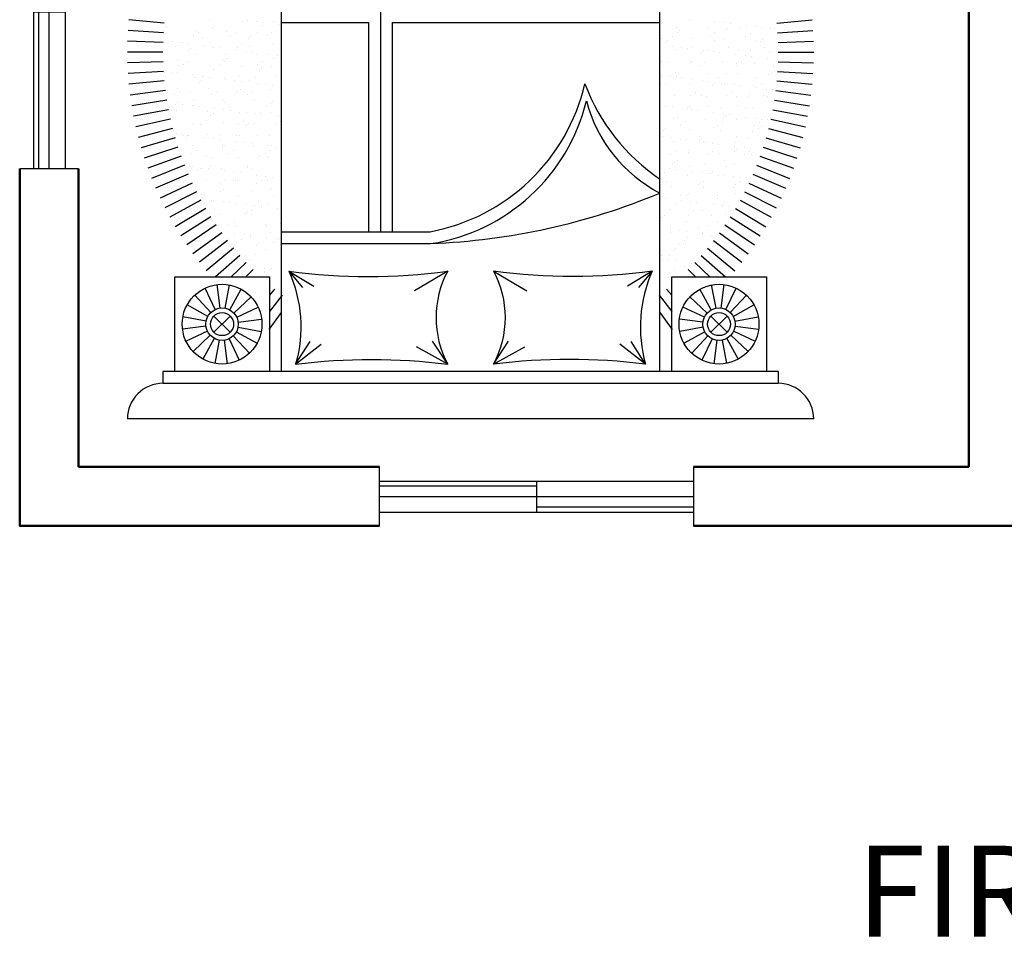
# Model space of a CAD drawing. Units: millimetres. Extents: x -857 to 54106, y -13666 to 13947.
# Tile 13 of 41: x 21020 to 24780, y 2329 to 5837. Entities that reach past the tile are written whole.
import ezdxf

# ---------------------------------------------------------------- set-up
doc = ezdxf.new("R2010")
doc.units = ezdxf.units.MM
for name, color, linetype, lineweight in [('A-ANNO-TEXT', 7, 'Continuous', 25), ('A-FURN', 21, 'Continuous', 18), ('A-GLAZ', 4, 'Continuous', 25), ('A-WALL', 7, 'Continuous', 50)]:
    doc.layers.add(name, color=color, linetype=linetype, lineweight=lineweight)
for name, color, linetype in [('A-FRN', 11, 'Continuous'), ('A-HT', 15, 'Continuous'), ('L-HT', 1, 'Continuous')]:
    doc.layers.add(name, color=color, linetype=linetype)
doc.styles.get("Standard").update_dxf_attribs({"font": 'arial.ttf'})

# ---------------------------------------------------------------- blocks, each defined once
blk = doc.blocks.new('*X18')
at = {"color": 0}
for p, q in [((0.9013, 1.6721), (0.9013, 1.6721)), ((0.9273, 1.6756), (0.9273, 1.6756)), ((0.9679, 1.6809), (0.9679, 1.6809)), ((1.075, 1.6828), (1.075, 1.6828)), ((2.8098, 1.6645), (2.8098, 1.6645)), ((2.8341, 1.6809), (2.8341, 1.6809)), ((2.8777, 1.6734), (2.8777, 1.6734)), ((2.9037, 1.6769), (2.9037, 1.6769)), ((2.9444, 1.6822), (2.9444, 1.6822)), ((2.962, 1.6803), (2.962, 1.6803)), ((3.0971, 1.6852), (3.0971, 1.6852)), ((0.7154, 1.6491), (0.7154, 1.6491)), ((0.7341, 1.6496), (0.7341, 1.6496)), ((0.7667, 1.6544), (0.7667, 1.6544)), ((0.7927, 1.6578), (0.7927, 1.6578)), ((0.8149, 1.6302), (0.8149, 1.6302)), ((0.8333, 1.6632), (0.8333, 1.6632)), ((0.865, 1.6513), (0.865, 1.6513)), ((0.9155, 1.6474), (0.9155, 1.6474)), ((0.9247, 1.6389), (0.9247, 1.6389)), ((0.9706, 1.6305), (0.9706, 1.6305)), ((0.9929, 1.6507), (0.9929, 1.6507)), ((1.1185, 1.6429), (1.1185, 1.6429)), ((1.1263, 1.6308), (1.1263, 1.6308)), ((1.1279, 1.6556), (1.1279, 1.6556)), ((2.8391, 1.6339), (2.8391, 1.6339)), ((2.8812, 1.6623), (2.8812, 1.6623)), ((2.9017, 1.634), (2.9017, 1.634)), ((2.9948, 1.6342), (2.9948, 1.6342)), ((3.0326, 1.6357), (3.0326, 1.6357)), ((3.0813, 1.6605), (3.0813, 1.6605)), ((3.0905, 1.6521), (3.0905, 1.6521)), ((3.1505, 1.6345), (3.1505, 1.6345)), ((3.1605, 1.6351), (3.1605, 1.6351)), ((3.2843, 1.6561), (3.2843, 1.6561)), ((3.2956, 1.64), (3.2956, 1.64)), ((0.7652, 1.6035), (0.7652, 1.6035)), ((0.7744, 1.595), (0.7744, 1.595)), ((0.7976, 1.5996), (0.7976, 1.5996)), ((0.836, 1.6168), (0.836, 1.6168)), ((0.9326, 1.6044), (0.9326, 1.6044)), ((0.9682, 1.599), (0.9682, 1.599)), ((0.9917, 1.6171), (0.9917, 1.6171)), ((1.0635, 1.6061), (1.0635, 1.6061)), ((1.1474, 1.6173), (1.1474, 1.6173)), ((1.1683, 1.5973), (1.1683, 1.5973)), ((1.1775, 1.5889), (1.1775, 1.5889)), ((1.1914, 1.6055), (1.1914, 1.6055)), ((2.8373, 1.5846), (2.8373, 1.5846)), ((2.8602, 1.6205), (2.8602, 1.6205)), ((2.931, 1.6167), (2.931, 1.6167)), ((2.9402, 1.6082), (2.9402, 1.6082)), ((2.9652, 1.584), (2.9652, 1.584)), ((3.0159, 1.6207), (3.0159, 1.6207)), ((3.1002, 1.5888), (3.1002, 1.5888)), ((3.134, 1.6122), (3.134, 1.6122)), ((3.1716, 1.621), (3.1716, 1.621)), ((3.193, 1.5855), (3.193, 1.5855)), ((3.219, 1.5889), (3.219, 1.5889)), ((3.2311, 1.5905), (3.2311, 1.5905)), ((3.2596, 1.5943), (3.2596, 1.5943)), ((0.7373, 1.5533), (0.7373, 1.5533)), ((0.7562, 1.5681), (0.7562, 1.5681)), ((0.8179, 1.5552), (0.8179, 1.5552)), ((0.8681, 1.555), (0.8681, 1.555)), ((0.8794, 1.5398), (0.8794, 1.5398)), ((0.9119, 1.5684), (0.9119, 1.5684)), ((0.9474, 1.5488), (0.9474, 1.5488)), ((0.9734, 1.5522), (0.9734, 1.5522)), ((0.996, 1.5544), (0.996, 1.5544)), ((1.014, 1.5575), (1.014, 1.5575)), ((1.018, 1.5534), (1.018, 1.5534)), ((1.0272, 1.545), (1.0272, 1.545)), ((1.0676, 1.5687), (1.0676, 1.5687)), ((1.0819, 1.5665), (1.0819, 1.5665)), ((1.108, 1.5699), (1.108, 1.5699)), ((1.1311, 1.5592), (1.1311, 1.5592)), ((1.1486, 1.5753), (1.1486, 1.5753)), ((2.8559, 1.5411), (2.8559, 1.5411)), ((2.9238, 1.55), (2.9238, 1.55)), ((2.9361, 1.5721), (2.9361, 1.5721)), ((2.9498, 1.5535), (2.9498, 1.5535)), ((2.9837, 1.5683), (2.9837, 1.5683)), ((2.9905, 1.5588), (2.9905, 1.5588)), ((3.0584, 1.5678), (3.0584, 1.5678)), ((3.0844, 1.5712), (3.0844, 1.5712)), ((3.0918, 1.5724), (3.0918, 1.5724)), ((3.1251, 1.5765), (3.1251, 1.5765)), ((3.1838, 1.5666), (3.1838, 1.5666)), ((3.193, 1.5582), (3.193, 1.5582)), ((3.2475, 1.5727), (3.2475, 1.5727)), ((3.2987, 1.5436), (3.2987, 1.5436)), ((0.7042, 1.5167), (0.7042, 1.5167)), ((0.7448, 1.5221), (0.7448, 1.5221)), ((0.8007, 1.5032), (0.8007, 1.5032)), ((0.8128, 1.531), (0.8128, 1.531)), ((0.8388, 1.5345), (0.8388, 1.5345)), ((0.8553, 1.505), (0.8553, 1.505)), ((0.8677, 1.5096), (0.8677, 1.5096)), ((0.8769, 1.5011), (0.8769, 1.5011)), ((0.9358, 1.5081), (0.9358, 1.5081)), ((1.011, 1.5053), (1.011, 1.5053)), ((1.0666, 1.5098), (1.0666, 1.5098)), ((1.0707, 1.5051), (1.0707, 1.5051)), ((1.1667, 1.5056), (1.1667, 1.5056)), ((1.1945, 1.5091), (1.1945, 1.5091)), ((2.8152, 1.5357), (2.8152, 1.5357)), ((2.8334, 1.5245), (2.8334, 1.5245)), ((2.8795, 1.5087), (2.8795, 1.5087)), ((2.9049, 1.5377), (2.9049, 1.5377)), ((3.0334, 1.5227), (3.0334, 1.5227)), ((3.0352, 1.509), (3.0352, 1.509)), ((3.0358, 1.5394), (3.0358, 1.5394)), ((3.0427, 1.5143), (3.0427, 1.5143)), ((3.1637, 1.5388), (3.1637, 1.5388)), ((3.1909, 1.5093), (3.1909, 1.5093)), ((3.2365, 1.5183), (3.2365, 1.5183)), ((0.7174, 1.4657), (0.7174, 1.4657)), ((0.7207, 1.4913), (0.7207, 1.4913)), ((0.7266, 1.4572), (0.7266, 1.4572)), ((0.7404, 1.457), (0.7404, 1.457)), ((0.8713, 1.4586), (0.8713, 1.4586)), ((0.8764, 1.4916), (0.8764, 1.4916)), ((0.9204, 1.4613), (0.9204, 1.4613)), ((0.9992, 1.458), (0.9992, 1.458)), ((1.0321, 1.4919), (1.0321, 1.4919)), ((1.1205, 1.4595), (1.1205, 1.4595)), ((1.1342, 1.4629), (1.1342, 1.4629)), ((1.1878, 1.4921), (1.1878, 1.4921)), ((2.8404, 1.4882), (2.8404, 1.4882)), ((2.8831, 1.4789), (2.8831, 1.4789)), ((2.8924, 1.4704), (2.8924, 1.4704)), ((2.9006, 1.4953), (2.9006, 1.4953)), ((2.9683, 1.4876), (2.9683, 1.4876)), ((3.0563, 1.4955), (3.0563, 1.4955)), ((3.0862, 1.4744), (3.0862, 1.4744)), ((3.1034, 1.4925), (3.1034, 1.4925)), ((3.212, 1.4958), (3.212, 1.4958)), ((3.2343, 1.4942), (3.2343, 1.4942)), ((3.2391, 1.4621), (3.2391, 1.4621)), ((3.2651, 1.4655), (3.2651, 1.4655)), ((3.2862, 1.4727), (3.2862, 1.4727)), ((3.2954, 1.4643), (3.2954, 1.4643)), ((0.7701, 1.4174), (0.7701, 1.4174)), ((0.7966, 1.4429), (0.7966, 1.4429)), ((0.9255, 1.4164), (0.9255, 1.4164)), ((0.9523, 1.4432), (0.9523, 1.4432)), ((0.9701, 1.4157), (0.9701, 1.4157)), ((0.9935, 1.4254), (0.9935, 1.4254)), ((1.0195, 1.4288), (1.0195, 1.4288)), ((1.0601, 1.4341), (1.0601, 1.4341)), ((1.108, 1.4435), (1.108, 1.4435)), ((1.128, 1.4431), (1.128, 1.4431)), ((1.1297, 1.4511), (1.1297, 1.4511)), ((1.1541, 1.4465), (1.1541, 1.4465)), ((1.1947, 1.4519), (1.1947, 1.4519)), ((2.8208, 1.4466), (2.8208, 1.4466)), ((2.902, 1.4177), (2.902, 1.4177)), ((2.908, 1.4414), (2.908, 1.4414)), ((2.9359, 1.4306), (2.9359, 1.4306)), ((2.9699, 1.4267), (2.9699, 1.4267)), ((2.9765, 1.4469), (2.9765, 1.4469)), ((2.9959, 1.4301), (2.9959, 1.4301)), ((3.0366, 1.4354), (3.0366, 1.4354)), ((3.0389, 1.443), (3.0389, 1.443)), ((3.1045, 1.4444), (3.1045, 1.4444)), ((3.1305, 1.4478), (3.1305, 1.4478)), ((3.1322, 1.4472), (3.1322, 1.4472)), ((3.1359, 1.4288), (3.1359, 1.4288)), ((3.1451, 1.4204), (3.1451, 1.4204)), ((3.1668, 1.4424), (3.1668, 1.4424)), ((3.1712, 1.4532), (3.1712, 1.4532)), ((3.2879, 1.4475), (3.2879, 1.4475)), ((0.7243, 1.3899), (0.7243, 1.3899)), ((0.74, 1.3795), (0.74, 1.3795)), ((0.7503, 1.3934), (0.7503, 1.3934)), ((0.7909, 1.3987), (0.7909, 1.3987)), ((0.8039, 1.4069), (0.8039, 1.4069)), ((0.8589, 1.4076), (0.8589, 1.4076)), ((0.8849, 1.4111), (0.8849, 1.4111)), ((0.8957, 1.3798), (0.8957, 1.3798)), ((0.9389, 1.4118), (0.9389, 1.4118)), ((0.9794, 1.4072), (0.9794, 1.4072)), ((1.0514, 1.3801), (1.0514, 1.3801)), ((1.0698, 1.4134), (1.0698, 1.4134)), ((1.1732, 1.4112), (1.1732, 1.4112)), ((1.1977, 1.4128), (1.1977, 1.4128)), ((2.8353, 1.4089), (2.8353, 1.4089)), ((2.8436, 1.3919), (2.8436, 1.3919)), ((2.8613, 1.4124), (2.8613, 1.4124)), ((2.9199, 1.3835), (2.9199, 1.3835)), ((2.9715, 1.3913), (2.9715, 1.3913)), ((2.9856, 1.385), (2.9856, 1.385)), ((2.9948, 1.3765), (2.9948, 1.3765)), ((3.0756, 1.3838), (3.0756, 1.3838)), ((3.1065, 1.3961), (3.1065, 1.3961)), ((3.1886, 1.3805), (3.1886, 1.3805)), ((3.2313, 1.384), (3.2313, 1.384)), ((3.2374, 1.3978), (3.2374, 1.3978)), ((0.7436, 1.3606), (0.7436, 1.3606)), ((0.761, 1.3661), (0.761, 1.3661)), ((0.8198, 1.3718), (0.8198, 1.3718)), ((0.8291, 1.3633), (0.8291, 1.3633)), ((0.8744, 1.3623), (0.8744, 1.3623)), ((0.9168, 1.3664), (0.9168, 1.3664)), ((1.0023, 1.3617), (1.0023, 1.3617)), ((1.0229, 1.3673), (1.0229, 1.3673)), ((1.0725, 1.3667), (1.0725, 1.3667)), ((1.1374, 1.3665), (1.1374, 1.3665)), ((2.8353, 1.3411), (2.8353, 1.3411)), ((2.8445, 1.3326), (2.8445, 1.3326)), ((2.9112, 1.345), (2.9112, 1.345)), ((2.9409, 1.37), (2.9409, 1.37)), ((3.0383, 1.3367), (3.0383, 1.3367)), ((3.0421, 1.3467), (3.0421, 1.3467)), ((3.0967, 1.3703), (3.0967, 1.3703)), ((3.17, 1.3461), (3.17, 1.3461)), ((3.2384, 1.3349), (3.2384, 1.3349)), ((3.2524, 1.3706), (3.2524, 1.3706)), ((0.807, 1.3105), (0.807, 1.3105)), ((0.837, 1.3177), (0.837, 1.3177)), ((0.8726, 1.3235), (0.8726, 1.3235)), ((0.9421, 1.3154), (0.9421, 1.3154)), ((0.9716, 1.293), (0.9716, 1.293)), ((0.9927, 1.318), (0.9927, 1.318)), ((1.0396, 1.302), (1.0396, 1.302)), ((1.0656, 1.3054), (1.0656, 1.3054)), ((1.0726, 1.3217), (1.0726, 1.3217)), ((1.0729, 1.3171), (1.0729, 1.3171)), ((1.0818, 1.3133), (1.0818, 1.3133)), ((1.1062, 1.3108), (1.1062, 1.3108)), ((1.1484, 1.3183), (1.1484, 1.3183)), ((1.1741, 1.3197), (1.1741, 1.3197)), ((2.8467, 1.2956), (2.8467, 1.2956)), ((2.8611, 1.3214), (2.8611, 1.3214)), ((2.888, 1.2928), (2.888, 1.2928)), ((2.9481, 1.2943), (2.9481, 1.2943)), ((2.9746, 1.2949), (2.9746, 1.2949)), ((3.016, 1.3033), (3.016, 1.3033)), ((3.0169, 1.3217), (3.0169, 1.3217)), ((3.042, 1.3067), (3.042, 1.3067)), ((3.0827, 1.312), (3.0827, 1.312)), ((3.0881, 1.291), (3.0881, 1.291)), ((3.1097, 1.2998), (3.1097, 1.2998)), ((3.1506, 1.321), (3.1506, 1.321)), ((3.1726, 1.322), (3.1726, 1.322)), ((3.1766, 1.3244), (3.1766, 1.3244)), ((3.2173, 1.3298), (3.2173, 1.3298)), ((3.2406, 1.3015), (3.2406, 1.3015)), ((3.2476, 1.3265), (3.2476, 1.3265)), ((0.7467, 1.2643), (0.7467, 1.2643)), ((0.7704, 1.2665), (0.7704, 1.2665)), ((0.7803, 1.2543), (0.7803, 1.2543)), ((0.7964, 1.27), (0.7964, 1.27)), ((0.837, 1.2753), (0.837, 1.2753)), ((0.8776, 1.2659), (0.8776, 1.2659)), ((0.905, 1.2843), (0.905, 1.2843)), ((0.9223, 1.2779), (0.9223, 1.2779)), ((0.931, 1.2877), (0.931, 1.2877)), ((0.9315, 1.2694), (0.9315, 1.2694)), ((0.936, 1.2546), (0.936, 1.2546)), ((1.0055, 1.2653), (1.0055, 1.2653)), ((1.0918, 1.2549), (1.0918, 1.2549)), ((1.1253, 1.2734), (1.1253, 1.2734)), ((1.1405, 1.2702), (1.1405, 1.2702)), ((2.8045, 1.258), (2.8045, 1.258)), ((2.8135, 1.2766), (2.8135, 1.2766)), ((2.8814, 1.2855), (2.8814, 1.2855)), ((2.9074, 1.289), (2.9074, 1.289)), ((2.9143, 1.2487), (2.9143, 1.2487)), ((2.9602, 1.2583), (2.9602, 1.2583)), ((3.0452, 1.2503), (3.0452, 1.2503)), ((3.0973, 1.2826), (3.0973, 1.2826)), ((3.1159, 1.2586), (3.1159, 1.2586)), ((3.1731, 1.2497), (3.1731, 1.2497)), ((0.772, 1.234), (0.772, 1.234)), ((0.7812, 1.2255), (0.7812, 1.2255)), ((0.8014, 1.2409), (0.8014, 1.2409)), ((0.8102, 1.2142), (0.8102, 1.2142)), ((0.9452, 1.2191), (0.9452, 1.2191)), ((0.9571, 1.2412), (0.9571, 1.2412)), ((0.975, 1.2296), (0.975, 1.2296)), ((1.0761, 1.2207), (1.0761, 1.2207)), ((1.1128, 1.2414), (1.1128, 1.2414)), ((1.1751, 1.2278), (1.1751, 1.2278)), ((1.1843, 1.2194), (1.1843, 1.2194)), ((2.8256, 1.2446), (2.8256, 1.2446)), ((2.9378, 1.2472), (2.9378, 1.2472)), ((2.947, 1.2387), (2.947, 1.2387)), ((2.9813, 1.2448), (2.9813, 1.2448)), ((3.137, 1.2451), (3.137, 1.2451)), ((3.1408, 1.2427), (3.1408, 1.2427)), ((0.8247, 1.1857), (0.8247, 1.1857)), ((0.8773, 1.1925), (0.8773, 1.1925)), ((0.8807, 1.1696), (0.8807, 1.1696)), ((1.0086, 1.169), (1.0086, 1.169)), ((1.0177, 1.1696), (1.0177, 1.1696)), ((1.0248, 1.184), (1.0248, 1.184)), ((1.033, 1.1928), (1.033, 1.1928)), ((1.034, 1.1755), (1.034, 1.1755)), ((1.0857, 1.1786), (1.0857, 1.1786)), ((1.1117, 1.182), (1.1117, 1.182)), ((1.1437, 1.1739), (1.1437, 1.1739)), ((1.1523, 1.1874), (1.1523, 1.1874)), ((1.1887, 1.1931), (1.1887, 1.1931)), ((2.8499, 1.1992), (2.8499, 1.1992)), ((2.9015, 1.1962), (2.9015, 1.1962)), ((2.9535, 1.1656), (2.9535, 1.1656)), ((2.9778, 1.1986), (2.9778, 1.1986)), ((2.9905, 1.1989), (2.9905, 1.1989)), ((2.9942, 1.1709), (2.9942, 1.1709)), ((3.0572, 1.1965), (3.0572, 1.1965)), ((3.0621, 1.1799), (3.0621, 1.1799)), ((3.0881, 1.1833), (3.0881, 1.1833)), ((3.1128, 1.2035), (3.1128, 1.2035)), ((3.1288, 1.1887), (3.1288, 1.1887)), ((3.1906, 1.1971), (3.1906, 1.1971)), ((3.1967, 1.1976), (3.1967, 1.1976)), ((3.1998, 1.1887), (3.1998, 1.1887)), ((3.2129, 1.1968), (3.2129, 1.1968)), ((3.2227, 1.201), (3.2227, 1.201)), ((3.2437, 1.2051), (3.2437, 1.2051)), ((0.8165, 1.1432), (0.8165, 1.1432)), ((0.8207, 1.1291), (0.8207, 1.1291)), ((0.8425, 1.1466), (0.8425, 1.1466)), ((0.8745, 1.1401), (0.8745, 1.1401)), ((0.8831, 1.1519), (0.8831, 1.1519)), ((0.8837, 1.1316), (0.8837, 1.1316)), ((0.9511, 1.1609), (0.9511, 1.1609)), ((0.9764, 1.1294), (0.9764, 1.1294)), ((0.9771, 1.1643), (0.9771, 1.1643)), ((1.0775, 1.1356), (1.0775, 1.1356)), ((1.0792, 1.1244), (1.0792, 1.1244)), ((1.1321, 1.1297), (1.1321, 1.1297)), ((2.8189, 1.1479), (2.8189, 1.1479)), ((2.8402, 1.155), (2.8402, 1.155)), ((2.8449, 1.1328), (2.8449, 1.1328)), ((2.8596, 1.1532), (2.8596, 1.1532)), ((2.9175, 1.1523), (2.9175, 1.1523)), ((2.9275, 1.1622), (2.9275, 1.1622)), ((3.0006, 1.1331), (3.0006, 1.1331)), ((3.0403, 1.1533), (3.0403, 1.1533)), ((3.0484, 1.154), (3.0484, 1.154)), ((3.0495, 1.1448), (3.0495, 1.1448)), ((3.1563, 1.1334), (3.1563, 1.1334)), ((3.1763, 1.1534), (3.1763, 1.1534)), ((0.8133, 1.1179), (0.8133, 1.1179)), ((0.8418, 1.1157), (0.8418, 1.1157)), ((0.9272, 1.0918), (0.9272, 1.0918)), ((0.9484, 1.1227), (0.9484, 1.1227)), ((0.9975, 1.116), (0.9975, 1.116)), ((1.1273, 1.09), (1.1273, 1.09)), ((1.1532, 1.1162), (1.1532, 1.1162)), ((2.853, 1.1029), (2.853, 1.1029)), ((2.866, 1.1194), (2.866, 1.1194)), ((2.89, 1.1094), (2.89, 1.1094)), ((2.8992, 1.1009), (2.8992, 1.1009)), ((2.9809, 1.1023), (2.9809, 1.1023)), ((3.0217, 1.1196), (3.0217, 1.1196)), ((3.093, 1.105), (3.093, 1.105)), ((3.116, 1.1071), (3.116, 1.1071)), ((3.1774, 1.1199), (3.1774, 1.1199)), ((0.8839, 1.0733), (0.8839, 1.0733)), ((0.9177, 1.0673), (0.9177, 1.0673)), ((0.977, 1.0462), (0.977, 1.0462)), ((1.0118, 1.0727), (1.0118, 1.0727)), ((1.0232, 1.0409), (1.0232, 1.0409)), ((1.0638, 1.0463), (1.0638, 1.0463)), ((1.0734, 1.0676), (1.0734, 1.0676)), ((1.1318, 1.0552), (1.1318, 1.0552)), ((1.1365, 1.0816), (1.1365, 1.0816)), ((1.1468, 1.0775), (1.1468, 1.0775)), ((1.1578, 1.0586), (1.1578, 1.0586)), ((1.18, 1.0417), (1.18, 1.0417)), ((1.1984, 1.064), (1.1984, 1.064)), ((2.9206, 1.056), (2.9206, 1.056)), ((2.9419, 1.071), (2.9419, 1.071)), ((2.9427, 1.0611), (2.9427, 1.0611)), ((2.9996, 1.0422), (2.9996, 1.0422)), ((3.0403, 1.0475), (3.0403, 1.0475)), ((3.0515, 1.0577), (3.0515, 1.0577)), ((3.0976, 1.0713), (3.0976, 1.0713)), ((3.1082, 1.0565), (3.1082, 1.0565)), ((3.1342, 1.0599), (3.1342, 1.0599)), ((3.1428, 1.0594), (3.1428, 1.0594)), ((3.152, 1.0509), (3.152, 1.0509)), ((3.1749, 1.0653), (3.1749, 1.0653)), ((3.1794, 1.057), (3.1794, 1.057)), ((0.8165, 1.0215), (0.8165, 1.0215)), ((0.8267, 1.0023), (0.8267, 1.0023)), ((0.8611, 1.0039), (0.8611, 1.0039)), ((0.8626, 1.0198), (0.8626, 1.0198)), ((0.8886, 1.0232), (0.8886, 1.0232)), ((0.9292, 1.0285), (0.9292, 1.0285)), ((0.9515, 1.0264), (0.9515, 1.0264)), ((0.9862, 1.0377), (0.9862, 1.0377)), ((0.9972, 1.0375), (0.9972, 1.0375)), ((1.0168, 1.0042), (1.0168, 1.0042)), ((1.0824, 1.0281), (1.0824, 1.0281)), ((1.1725, 1.0045), (1.1725, 1.0045)), ((2.839, 1.0211), (2.839, 1.0211)), ((2.8562, 1.0065), (2.8562, 1.0065)), ((2.865, 1.0245), (2.865, 1.0245)), ((2.8853, 1.0076), (2.8853, 1.0076)), ((2.9057, 1.0298), (2.9057, 1.0298)), ((2.9736, 1.0388), (2.9736, 1.0388)), ((2.9841, 1.0059), (2.9841, 1.0059)), ((2.9925, 1.0155), (2.9925, 1.0155)), ((3.0017, 1.007), (3.0017, 1.007)), ((3.041, 1.0079), (3.041, 1.0079)), ((3.1191, 1.0108), (3.1191, 1.0108)), ((0.8359, 0.9938), (0.8359, 0.9938)), ((0.8822, 0.9905), (0.8822, 0.9905)), ((0.887, 0.9769), (0.887, 0.9769)), ((1.0149, 0.9763), (1.0149, 0.9763)), ((1.0297, 0.9979), (1.0297, 0.9979)), ((1.0379, 0.9908), (1.0379, 0.9908)), ((1.15, 0.9812), (1.15, 0.9812)), ((1.1936, 0.991), (1.1936, 0.991)), ((2.8421, 0.9716), (2.8421, 0.9716)), ((2.8514, 0.9631), (2.8514, 0.9631)), ((2.9064, 0.9942), (2.9064, 0.9942)), ((2.9238, 0.9597), (2.9238, 0.9597)), ((3.0452, 0.9672), (3.0452, 0.9672)), ((3.0547, 0.9613), (3.0547, 0.9613)), ((3.0621, 0.9944), (3.0621, 0.9944)), ((0.8794, 0.954), (0.8794, 0.954)), ((0.9546, 0.93), (0.9546, 0.93)), ((0.9581, 0.9421), (0.9581, 0.9421)), ((1.0693, 0.9175), (1.0693, 0.9175)), ((1.0795, 0.9523), (1.0795, 0.9523)), ((1.0855, 0.9317), (1.0855, 0.9317)), ((1.0887, 0.9438), (1.0887, 0.9438)), ((1.1099, 0.9229), (1.1099, 0.9229)), ((1.1138, 0.9424), (1.1138, 0.9424)), ((1.1779, 0.9318), (1.1779, 0.9318)), ((2.8266, 0.9455), (2.8266, 0.9455)), ((2.8949, 0.9233), (2.8949, 0.9233)), ((2.9823, 0.9458), (2.9823, 0.9458)), ((3.0457, 0.9188), (3.0457, 0.9188)), ((3.0864, 0.9242), (3.0864, 0.9242)), ((3.0949, 0.9216), (3.0949, 0.9216)), ((3.138, 0.9461), (3.138, 0.9461)), ((0.8902, 0.8806), (0.8902, 0.8806)), ((0.9015, 0.8787), (0.9015, 0.8787)), ((0.9087, 0.8964), (0.9087, 0.8964)), ((0.9292, 0.9084), (0.9292, 0.9084)), ((0.9347, 0.8998), (0.9347, 0.8998)), ((0.9384, 0.8999), (0.9384, 0.8999)), ((0.9753, 0.9052), (0.9753, 0.9052)), ((1.0181, 0.88), (1.0181, 0.88)), ((1.0433, 0.9141), (1.0433, 0.9141)), ((1.0572, 0.879), (1.0572, 0.879)), ((1.1322, 0.904), (1.1322, 0.904)), ((1.1531, 0.8848), (1.1531, 0.8848)), ((2.8172, 0.8887), (2.8172, 0.8887)), ((2.8593, 0.9102), (2.8593, 0.9102)), ((2.8851, 0.8977), (2.8851, 0.8977)), ((2.9111, 0.9011), (2.9111, 0.9011)), ((2.9257, 0.8824), (2.9257, 0.8824)), ((2.9446, 0.8777), (2.9446, 0.8777)), ((2.9518, 0.9064), (2.9518, 0.9064)), ((2.9872, 0.9096), (2.9872, 0.9096)), ((3.0197, 0.9154), (3.0197, 0.9154)), ((3.0814, 0.8827), (3.0814, 0.8827)), ((3.1041, 0.9131), (3.1041, 0.9131)), ((3.1223, 0.9144), (3.1223, 0.9144)), ((0.9226, 0.8653), (0.9226, 0.8653)), ((0.9578, 0.8337), (0.9578, 0.8337)), ((0.9819, 0.8601), (0.9819, 0.8601)), ((1.0783, 0.8655), (1.0783, 0.8655)), ((1.0887, 0.8354), (1.0887, 0.8354)), ((1.1819, 0.8583), (1.1819, 0.8583)), ((1.1912, 0.8499), (1.1912, 0.8499)), ((2.9269, 0.8633), (2.9269, 0.8633)), ((2.9468, 0.8689), (2.9468, 0.8689)), ((2.9538, 0.8692), (2.9538, 0.8692)), ((3.0578, 0.865), (3.0578, 0.865)), ((3.1025, 0.8692), (3.1025, 0.8692)), ((0.9985, 0.8169), (0.9985, 0.8169)), ((1.0316, 0.8145), (1.0316, 0.8145)), ((1.0409, 0.806), (1.0409, 0.806)), ((1.0894, 0.7907), (1.0894, 0.7907)), ((1.1154, 0.7941), (1.1154, 0.7941)), ((1.1542, 0.8172), (1.1542, 0.8172)), ((1.156, 0.7995), (1.156, 0.7995)), ((2.8035, 0.8253), (2.8035, 0.8253)), ((2.8625, 0.8138), (2.8625, 0.8138)), ((2.867, 0.8203), (2.867, 0.8203)), ((2.9904, 0.8132), (2.9904, 0.8132)), ((2.9973, 0.8294), (2.9973, 0.8294)), ((3.0227, 0.8206), (3.0227, 0.8206)), ((0.9808, 0.7764), (0.9808, 0.7764)), ((1.0212, 0.7836), (1.0212, 0.7836)), ((1.0214, 0.7818), (1.0214, 0.7818)), ((1.0844, 0.7662), (1.0844, 0.7662)), ((1.0976, 0.7538), (1.0976, 0.7538)), ((1.1563, 0.7885), (1.1563, 0.7885)), ((2.8104, 0.7569), (2.8104, 0.7569)), ((2.8227, 0.76), (2.8227, 0.76)), ((2.847, 0.7855), (2.847, 0.7855)), ((2.8633, 0.7653), (2.8633, 0.7653)), ((2.9301, 0.767), (2.9301, 0.767)), ((2.9312, 0.7743), (2.9312, 0.7743)), ((2.9572, 0.7777), (2.9572, 0.7777)), ((2.9661, 0.7572), (2.9661, 0.7572)), ((2.9979, 0.7831), (2.9979, 0.7831)), ((3.0471, 0.7838), (3.0471, 0.7838)), ((1.0918, 0.739), (1.0918, 0.739)), ((1.1187, 0.7403), (1.1187, 0.7403)), ((1.1341, 0.7206), (1.1341, 0.7206)), ((1.1433, 0.7121), (1.1433, 0.7121)), ((2.8314, 0.7435), (2.8314, 0.7435)), ((2.8656, 0.7175), (2.8656, 0.7175)), ((2.8968, 0.7399), (2.8968, 0.7399)), ((2.906, 0.7314), (2.906, 0.7314)), ((2.9871, 0.7437), (2.9871, 0.7437)), ((2.9935, 0.7169), (2.9935, 0.7169)), ((1.0389, 0.6917), (1.0389, 0.6917)), ((1.1355, 0.6673), (1.1355, 0.6673)), ((1.1594, 0.6922), (1.1594, 0.6922)), ((1.1615, 0.6707), (1.1615, 0.6707)), ((1.1868, 0.6723), (1.1868, 0.6723)), ((1.1946, 0.692), (1.1946, 0.692)), ((2.9073, 0.6951), (2.9073, 0.6951)), ((2.9332, 0.6706), (2.9332, 0.6706)), ((2.9495, 0.6916), (2.9495, 0.6916)), ((1.0675, 0.6584), (1.0675, 0.6584)), ((1.095, 0.6427), (1.095, 0.6427)), ((1.138, 0.6286), (1.138, 0.6286)), ((2.8427, 0.6332), (2.8427, 0.6332)), ((2.8507, 0.6317), (2.8507, 0.6317)), ((2.8688, 0.6366), (2.8688, 0.6366)), ((2.9094, 0.6419), (2.9094, 0.6419)), ((1.159, 0.6151), (1.159, 0.6151)), ((1.1626, 0.5958), (1.1626, 0.5958)), ((2.849, 0.6021), (2.849, 0.6021)), ((2.8688, 0.6212), (2.8688, 0.6212)), ((2.8718, 0.6183), (2.8718, 0.6183)), ((1.1816, 0.5439), (1.1816, 0.5439)), ((2.8013, 0.5694), (2.8013, 0.5694))]:
    blk.add_line(p, q, dxfattribs=at)
blk = doc.blocks.new('A$C6796526C')
at = {"layer": 'A-FRN'}
for p, q in [((0, 3), (2.9, 3)), ((2.75, 2.85), (0.15, 2.85)), ((0.15, 2.8), (0.15, 2.85)), ((2.75, 2.8), (2.75, 2.85)), ((0.15, 2.8), (2.75, 2.8)), ((0.2, 2.4), (0.2, 2.8)), ((0.6, 2.8), (0.6, 2.4)), ((2.3, 2.4), (2.3, 2.8)), ((2.7, 2.8), (2.7, 2.4)), ((0.6, 2.4), (0.2, 2.4)), ((2.7, 2.4), (2.3, 2.4))]:
    blk.add_line(p, q, dxfattribs=at)
blk.add_lwpolyline([(0.65, 2.8), (0.65, 0.9), (2.25, 0.9), (2.25, 2.8)], dxfattribs=at)
for points in [[(0.6821, 2.3755, 0.175461), (0.7109, 2.7686)], [(0.7109, 2.7686, 0.059544), (1.3533, 2.7686)], [(1.3533, 2.3755, -0.248743), (1.3533, 2.7686)], [(2.1891, 2.7686, -0.059544), (1.5467, 2.7686)], [(1.5467, 2.3755, 0.248743), (1.5467, 2.7686)], [(2.2179, 2.3755, -0.175461), (2.1891, 2.7686)], [(0.6821, 2.3755, -0.069628), (1.3533, 2.3755)], [(2.2179, 2.3755, 0.069628), (1.5467, 2.3755)], [(2.25, 2.2594), (1.6173, 2.2594, 0.303651), (0.9607, 1.6568, 0.210515), (0.65, 2.0462)]]:
    blk.add_lwpolyline(points, format="xyb", dxfattribs=at)
for centre, radius in [((0.4, 2.6), 0.1686), ((2.5, 2.6), 0.1686), ((0.4, 2.6), 0.0686), ((2.5, 2.6), 0.0686)]:
    blk.add_circle(centre, radius, dxfattribs=at)
for centre, radius, start, end in [((0.15, 3), 0.15, 180, 270), ((2.75, 3), 0.15, 270, 0), ((1.7313, -0.5592), 2.8209, 92.3174, 112.5397)]:
    blk.add_arc(centre, radius, start, end, dxfattribs=at)
at = {"layer": 'A-HT'}
for p, q in [((0.65, 2.5511), (0.5977, 2.6231)), ((2.25, 2.5511), (2.3023, 2.6231)), ((0.6532, 2.4772), (0.6, 2.5458)), ((2.2468, 2.4772), (2.3, 2.5458)), ((0.6213, 2.4517), (0.6, 2.4775)), ((2.2787, 2.4517), (2.3, 2.4775)), ((0.4483, 2.2787), (0.3328, 2.3743)), ((0.4749, 2.3097), (0.3724, 2.4)), ((0.5023, 2.3399), (0.4384, 2.4)), ((0.5308, 2.3692), (0.5, 2.4)), ((2.3692, 2.3692), (2.4, 2.4)), ((2.3977, 2.3399), (2.4616, 2.4)), ((2.4251, 2.3097), (2.5276, 2.4)), ((2.4517, 2.2787), (2.5672, 2.3743)), ((0.4228, 2.2468), (0.3043, 2.3387)), ((2.4772, 2.2468), (2.5957, 2.3387)), ((0.3983, 2.2141), (0.2769, 2.3023)), ((2.5017, 2.2141), (2.6231, 2.3023)), ((0.3748, 2.1807), (0.2507, 2.265)), ((2.5252, 2.1807), (2.6493, 2.265)), ((0.3524, 2.1466), (0.2257, 2.2269)), ((2.5476, 2.1466), (2.6743, 2.2269)), ((0.331, 2.1118), (0.2019, 2.1881)), ((2.569, 2.1118), (2.6981, 2.1881)), ((0.3108, 2.0763), (0.1794, 2.1485)), ((2.5892, 2.0763), (2.7206, 2.1485)), ((0.2917, 2.0402), (0.158, 2.1083)), ((2.6083, 2.0402), (2.742, 2.1083)), ((0.2737, 2.0035), (0.138, 2.0674)), ((2.6263, 2.0035), (2.762, 2.0674)), ((0.2569, 1.9663), (0.1193, 2.0259)), ((2.6431, 1.9663), (2.7807, 2.0259)), ((0.2413, 1.9286), (0.1018, 1.9838)), ((2.6587, 1.9286), (2.7982, 1.9838)), ((0.2269, 1.8904), (0.0857, 1.9412)), ((2.6731, 1.8904), (2.8143, 1.9412)), ((0.2136, 1.8517), (0.071, 1.8981)), ((2.6864, 1.8517), (2.829, 1.8981)), ((0.2016, 1.8127), (0.0576, 1.8545)), ((2.6984, 1.8127), (2.8424, 1.8545)), ((0.1908, 1.7733), (0.0456, 1.8106)), ((2.7092, 1.7733), (2.8544, 1.8106)), ((0.1813, 1.7336), (0.0349, 1.7663)), ((2.7187, 1.7336), (2.8651, 1.7663)), ((0.173, 1.6936), (0.0257, 1.7217)), ((2.727, 1.6936), (2.8743, 1.7217)), ((0.166, 1.6534), (0.0179, 1.6768)), ((2.734, 1.6534), (2.8821, 1.6768)), ((0.1603, 1.6129), (0.0114, 1.6317)), ((2.7397, 1.6129), (2.8886, 1.6317)), ((0.1558, 1.5723), (0.0064, 1.5865)), ((2.7442, 1.5723), (2.8936, 1.5865)), ((0.1526, 1.5316), (0.0029, 1.541)), ((2.7474, 1.5316), (2.8971, 1.541)), ((0.1506, 1.4908), (0.0007, 1.4955)), ((2.7494, 1.4908), (2.8993, 1.4955)), ((0.15, 1.45), (0, 1.45)), ((2.75, 1.45), (2.9, 1.45)), ((0.1506, 1.4092), (0.0007, 1.4045)), ((2.7494, 1.4092), (2.8993, 1.4045)), ((0.1526, 1.3684), (0.0029, 1.359)), ((2.7474, 1.3684), (2.8971, 1.359)), ((0.1558, 1.3277), (0.0064, 1.3135)), ((2.7442, 1.3277), (2.8936, 1.3135))]:
    blk.add_line(p, q, dxfattribs=at)
at = {"layer": 'L-HT'}
for p, q in [((0.3671, 2.6601), (0.319, 2.7478)), ((0.3873, 2.6674), (0.3687, 2.7656)), ((0.4087, 2.668), (0.4214, 2.7672)), ((0.4293, 2.662), (0.472, 2.7524)), ((0.7109, 2.7686), (0.8188, 2.6839)), ((0.7109, 2.7686), (0.7717, 2.6727)), ((1.3533, 2.7686), (1.2212, 2.6952)), ((1.3533, 2.7686), (1.2893, 2.6715)), ((1.5467, 2.7686), (1.6107, 2.6715)), ((1.5467, 2.7686), (1.6788, 2.6952)), ((2.1891, 2.7686), (2.0812, 2.6839)), ((2.1891, 2.7686), (2.1283, 2.6727)), ((2.4707, 2.662), (2.428, 2.7524)), ((2.4913, 2.668), (2.4786, 2.7672)), ((2.5127, 2.6674), (2.5313, 2.7656)), ((2.5329, 2.6601), (2.581, 2.7478)), ((0.3501, 2.647), (0.2773, 2.7156)), ((0.447, 2.6499), (0.5156, 2.7227)), ((2.453, 2.6499), (2.3844, 2.7227)), ((2.5499, 2.647), (2.6227, 2.7156)), ((0.338, 2.6293), (0.2476, 2.672)), ((0.4601, 2.6329), (0.5478, 2.681)), ((2.4399, 2.6329), (2.3522, 2.681)), ((2.562, 2.6293), (2.6524, 2.672)), ((0.332, 2.6087), (0.2328, 2.6214)), ((0.3657, 2.5657), (0.4343, 2.6343)), ((0.4343, 2.5657), (0.3657, 2.6343)), ((0.4674, 2.6127), (0.5656, 2.6313)), ((2.4326, 2.6127), (2.3344, 2.6313)), ((2.4657, 2.5657), (2.5343, 2.6343)), ((2.5343, 2.5657), (2.4657, 2.6343)), ((2.568, 2.6087), (2.6672, 2.6214)), ((0.3326, 2.5873), (0.2344, 2.5687)), ((0.468, 2.5913), (0.5672, 2.5786)), ((2.432, 2.5913), (2.3328, 2.5786)), ((2.5674, 2.5873), (2.6656, 2.5687)), ((0.3399, 2.5671), (0.2522, 2.519)), ((0.353, 2.5501), (0.2844, 2.4773)), ((0.4329, 2.5399), (0.481, 2.4522)), ((0.4499, 2.553), (0.5227, 2.4844)), ((0.462, 2.5707), (0.5524, 2.528)), ((2.438, 2.5707), (2.3476, 2.528)), ((2.4501, 2.553), (2.3773, 2.4844)), ((2.4671, 2.5399), (2.419, 2.4522)), ((2.547, 2.5501), (2.6156, 2.4773)), ((2.5601, 2.5671), (2.6478, 2.519)), ((0.3707, 2.538), (0.328, 2.4476)), ((0.3913, 2.532), (0.3786, 2.4328)), ((0.4127, 2.5326), (0.4313, 2.4344)), ((2.4873, 2.5326), (2.4687, 2.4344)), ((2.5087, 2.532), (2.5214, 2.4328)), ((2.5293, 2.538), (2.572, 2.4476)), ((1.3533, 2.3755), (1.2125, 2.4585)), ((1.5467, 2.3755), (1.6875, 2.4585)), ((0.6821, 2.3755), (0.7405, 2.4447)), ((0.6821, 2.3755), (0.7872, 2.4395)), ((2.2179, 2.3755), (2.1128, 2.4395)), ((2.2179, 2.3755), (2.1595, 2.4447)), ((2.25, 2.2094), (1.6212, 2.2094)), ((1.7809, 1.3249), (1.7809, 2.2094)), ((1.8309, 0.9), (1.8309, 2.2094)), ((1.8809, 1.3249), (1.8809, 2.2094)), ((1.7809, 1.3249), (0.65, 1.3249)), ((2.25, 1.3249), (1.8809, 1.3249))]:
    blk.add_line(p, q, dxfattribs=at)
for centre in [(0.4, 2.6), (2.5, 2.6)]:
    blk.add_circle(centre, 0.0486, dxfattribs=at)
for centre, radius, start, end in [((1.7721, 1.396), 0.8272, 100.5107, 166.872), ((0.1786, 1.2908), 0.8406, 20.4105, 55.8901)]:
    blk.add_arc(centre, radius, start, end, dxfattribs=at)
at = {"layer": 'A-HT', "extrusion": (0, 0, -1), "zscale": -1, "rotation": 180}
blk.add_blockref('*X18', (0.55, 3), dxfattribs=at)
blk = doc.blocks.new('WIN-1200')
for p, q in [((9371.3, 11750.2), (10571.3, 11750.2)), ((9371.3, 11731.7), (9971.3, 11731.7)), ((9971.3, 11750.2), (9971.3, 11630.7)), ((9371.3, 11691.7), (10571.3, 11691.7)), ((10571.3, 11630.7), (9371.3, 11630.7)), ((9971.3, 11651.7), (10571.3, 11651.7))]:
    blk.add_line(p, q)
for points in [[(9371.3, 11579.2), (9371.3, 11804.2)], [(10571.3, 11804.2), (10571.3, 11579.2)]]:
    blk.add_lwpolyline(points)

msp = doc.modelspace()

# ---------------------------------------------------------------- linework, layer by layer
at = {"layer": 'A-WALL'}
for p, q in [((24645.079, 7729.231), (24645.079, 4129.231)), ((21245.079, 4129.231), (21245.079, 5267.586)), ((21245.079, 4129.231), (22393.518, 4129.231)), ((23593.518, 4129.023), (24645.079, 4129.231)), ((23593.518, 3904.023), (24870.079, 3904.023))]:
    msp.add_line(p, q, dxfattribs=at)
msp.add_lwpolyline([(22393.518, 3904.094), (21020.079, 3904.258), (21020.079, 5267.586)], dxfattribs=at)

# ---------------------------------------------------------------- block references
at = {"layer": 'A-FURN', "xscale": 903.6084929786902, "yscale": 903.6084929786902, "zscale": 903.6084929786902, "rotation": 179.9999999999989}
msp.add_blockref('A$C6796526C', (24051.97, 7023.692), dxfattribs=at)
at = {"layer": 'A-GLAZ', "rotation": 90.00000000000063}
msp.add_blockref('WIN-1200', (32824.31, -4103.754), dxfattribs=at)
at = {"layer": 'A-GLAZ'}
msp.add_blockref('WIN-1200', (13022.177, -7675.208), dxfattribs=at)

# ---------------------------------------------------------------- texts
at = {"layer": 'A-ANNO-TEXT', "insert": (24215.858, 2682.963), "char_height": 347.60543, "attachment_point": 1}
msp.add_mtext_dynamic_manual_height_columns('\\pxt0;FIRST FLOOR PLAN', width=5900.0263, gutter_width=43450.679, heights=[5996.136], dxfattribs=at)

doc.saveas('drawing.dxf')
